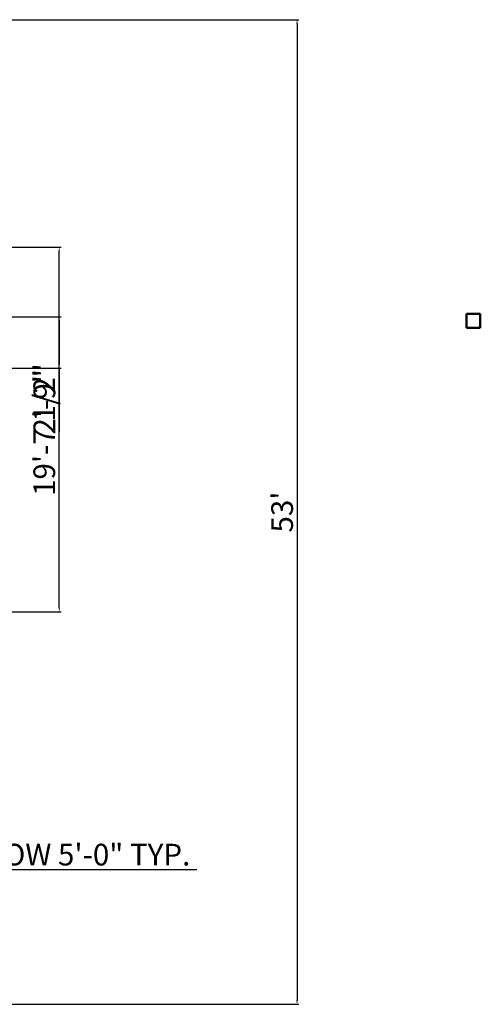
# Model space of a CAD drawing. Units: inches. Extents: x 3316 to 4157, y 2203 to 2977.
# Tile 4 of 4: x 3860 to 4157, y 2252 to 2888. Entities that reach past the tile are written whole.
import ezdxf

# ---------------------------------------------------------------- set-up
doc = ezdxf.new("R2010")
doc.units = ezdxf.units.IN
doc.layers.add('A-ANNO-DIMS', color=2, linetype='Continuous', lineweight=18)
doc.layers.add('A-COLS', color=7, linetype='Continuous', lineweight=50)
doc.styles.get("Standard").update_dxf_attribs({"font": 'arial.ttf'})
doc.dimstyles.new('ISO-25', dxfattribs={"dimtxt": 14, "dimasz": 2.5, "dimexe": 1.25, "dimexo": 0.625, "dimtad": 1, "dimlunit": 3, "dimtxsty": 'Standard', "dimcen": 2.5, "dimadec": 0, "dimazin": 0, "dimtfac": 1, "dimtmove": 0, "dimatfit": 3, "dimfxl": 1, "dimarcsym": 0})

# ---------------------------------------------------------------- blocks, each defined once
blk = doc.blocks.new('*D7')
at = {"layer": 'A-ANNO-DIMS', "color": 0, "lineweight": -2, "transparency": 16777216}
for p, q in [((3850.21, 2887.84), (4040.36, 2887.84)), ((4039.11, 2885.34), (4039.11, 2254.34)), ((3850.21, 2251.84), (4040.36, 2251.84))]:
    blk.add_line(p, q, dxfattribs=at)
at = {"layer": 'A-ANNO-DIMS', "color": 0, "transparency": 16777216}
for points in [[(4038.69, 2885.34), (4039.53, 2885.34), (4039.11, 2887.84)], [(4038.69, 2254.34), (4039.53, 2254.34), (4039.11, 2251.84)]]:
    blk.add_solid(points, dxfattribs=at)
at = {"layer": 'Defpoints', "color": 0, "transparency": 16777216}
for p in [(3849.58, 2887.84), (3849.58, 2251.84), (4039.11, 2251.84)]:
    blk.add_point(p, dxfattribs=at)
at = {"layer": 'A-ANNO-DIMS', "color": 0, "transparency": 16777216, "insert": (4031.33, 2569.84), "char_height": 14, "attachment_point": 5, "rotation": 90}
blk.add_mtext("53'", dxfattribs=at)
blk = doc.blocks.new('COL-9IN-SQ')
for p, q in [((0, 9), (0, 0)), ((9, 9), (0, 9)), ((9, 0), (9, 9)), ((0, 0), (9, 0))]:
    blk.add_line(p, q)
blk = doc.blocks.new('*D38')
at = {"layer": 'A-ANNO-DIMS', "color": 0, "lineweight": -2, "transparency": 16777216}
for p, q in [((3733.56, 2347.22), (3733.56, 2337.59)), ((3793.56, 2347.22), (3793.56, 2337.59)), ((3736.06, 2338.84), (3791.06, 2338.84)), ((3793.56, 2338.84), (3974.47, 2338.84))]:
    blk.add_line(p, q, dxfattribs=at)
at = {"layer": 'A-ANNO-DIMS', "color": 0, "transparency": 16777216}
for points in [[(3736.06, 2339.26), (3736.06, 2338.43), (3733.56, 2338.84)], [(3791.06, 2339.26), (3791.06, 2338.43), (3793.56, 2338.84)]]:
    blk.add_solid(points, dxfattribs=at)
at = {"layer": 'Defpoints', "color": 0, "transparency": 16777216}
for p in [(3733.56, 2347.84), (3793.56, 2347.84), (3793.56, 2338.84)]:
    blk.add_point(p, dxfattribs=at)
at = {"layer": 'A-ANNO-DIMS', "color": 0, "transparency": 16777216, "insert": (3885.26, 2346.71), "char_height": 14, "attachment_point": 5}
blk.add_mtext('WINDOW 5\'-0" TYP.', dxfattribs=at)
blk = doc.blocks.new('*D51')
at = {"layer": 'A-ANNO-DIMS', "color": 0, "lineweight": -2, "transparency": 16777216}
for p, q in [((3562.21, 2695.84), (3886.88, 2695.84)), ((3885.63, 2693.34), (3885.63, 2665.34)), ((3562.21, 2662.84), (3886.88, 2662.84)), ((3885.63, 2662.84), (3885.63, 2621.64))]:
    blk.add_line(p, q, dxfattribs=at)
at = {"layer": 'A-ANNO-DIMS', "color": 0, "transparency": 16777216}
for points in [[(3885.22, 2693.34), (3886.05, 2693.34), (3885.63, 2695.84)], [(3885.22, 2665.34), (3886.05, 2665.34), (3885.63, 2662.84)]]:
    blk.add_solid(points, dxfattribs=at)
at = {"layer": 'Defpoints', "color": 0, "transparency": 16777216}
for p in [(3561.58, 2695.84), (3561.58, 2662.84), (3885.63, 2662.84)]:
    blk.add_point(p, dxfattribs=at)
at = {"layer": 'A-ANNO-DIMS', "color": 0, "transparency": 16777216, "insert": (3877.86, 2640.99), "char_height": 14, "attachment_point": 5, "rotation": 90}
blk.add_mtext('2\'-9"', dxfattribs=at)
blk = doc.blocks.new('*D57')
at = {"layer": 'A-ANNO-DIMS', "color": 0, "lineweight": -2, "transparency": 16777216}
for p, q in [((3692.71, 2740.84), (3886.88, 2740.84)), ((3885.63, 2507.84), (3885.63, 2738.34)), ((3676.19, 2505.34), (3886.88, 2505.34))]:
    blk.add_line(p, q, dxfattribs=at)
at = {"layer": 'A-ANNO-DIMS', "color": 0, "transparency": 16777216}
for points in [[(3885.22, 2738.34), (3886.05, 2738.34), (3885.63, 2740.84)], [(3885.22, 2507.84), (3886.05, 2507.84), (3885.63, 2505.34)]]:
    blk.add_solid(points, dxfattribs=at)
at = {"layer": 'Defpoints', "color": 0, "transparency": 16777216}
for p in [(3692.08, 2740.84), (3885.63, 2740.84), (3675.57, 2505.34)]:
    blk.add_point(p, dxfattribs=at)
at = {"layer": 'A-ANNO-DIMS', "color": 0, "transparency": 16777216, "insert": (3877.77, 2623.09), "char_height": 14, "attachment_point": 5, "rotation": 90}
blk.add_mtext('19\'-7 1/2"', dxfattribs=at)

msp = doc.modelspace()

# ---------------------------------------------------------------- block references
at = {"layer": 'A-COLS'}
msp.add_blockref('COL-9IN-SQ', (4148.427, 2688.888), dxfattribs=at)

# ---------------------------------------------------------------- dimensions: what is measured, and where the dimension line sits
at = {"layer": 'A-ANNO-DIMS'}
for base, p1, p2, override, picture, middle in [((4039.111, 2251.842), (3849.584, 2887.842), (3849.584, 2251.842), {"dimclrd": 0, "dimclre": 0, "dimclrt": 0}, '*D7', (4031.333, 2569.842)), ((3885.634, 2740.842), (3675.569, 2505.342), (3692.084, 2740.842), {"dimdec": 1, "dimlfac": 1, "dimrnd": 0, "dimzin": 1, "dimdsep": 46, "dimlunit": 4, "dimfrac": 2}, '*D57', (3877.77, 2623.092)), ((3885.634, 2662.842), (3561.584, 2695.842), (3561.584, 2662.842), {"dimdec": 1, "dimlfac": 1, "dimrnd": 0, "dimzin": 1, "dimdsep": 46, "dimlunit": 4, "dimfrac": 2}, '*D51', (3877.861, 2640.99))]:
    dim = msp.add_linear_dim(base=base, p1=p1, p2=p2, angle=90, dimstyle='ISO-25', override=override, dxfattribs=at)
    dim.commit()
    dim.dimension.update_dxf_attribs({"geometry": picture, "text_midpoint": middle})
dim = msp.add_linear_dim(base=(3793.559, 2338.842), p1=(3733.559, 2347.842), p2=(3793.559, 2347.842), text='WINDOW <> TYP.', dimstyle='ISO-25', override={"dimdec": 1, "dimlfac": 1, "dimrnd": 0, "dimzin": 1, "dimdsep": 46, "dimlunit": 4, "dimfrac": 2}, dxfattribs=at)
dim.commit()
dim.dimension.update_dxf_attribs({"geometry": '*D38', "text_midpoint": (3885.263, 2346.711)})

doc.saveas('drawing.dxf')
